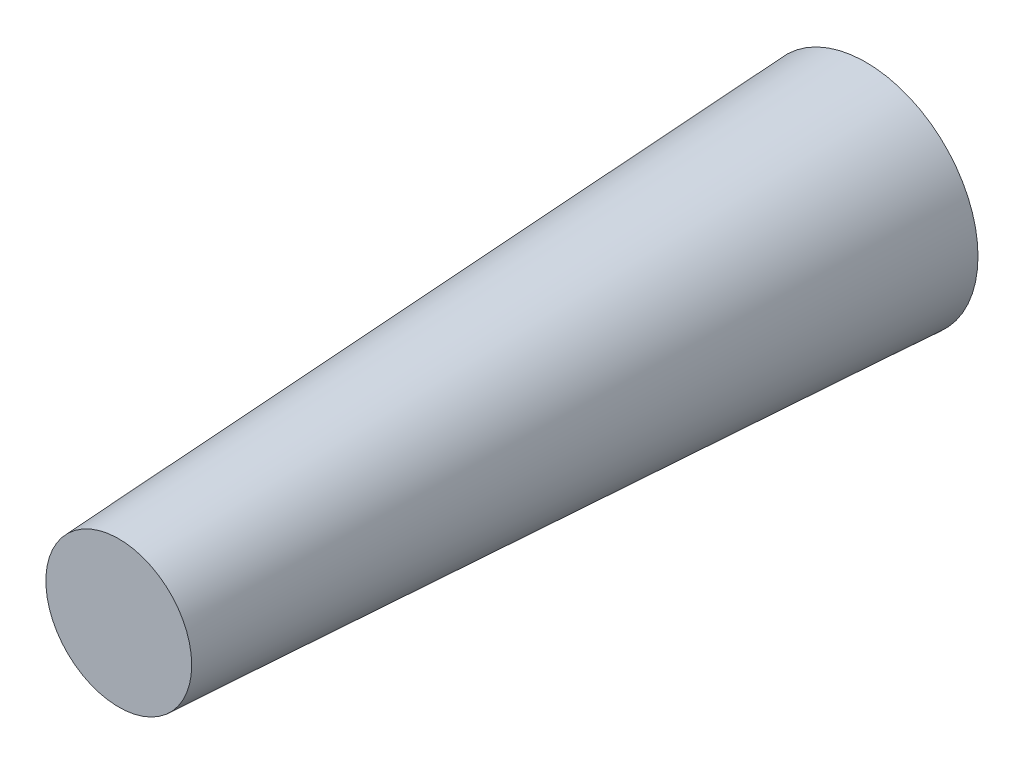
from build123d import *

# Parameters (mm, degrees)
PIN_PROFILE_6_R                   = 3
TAPER_PIN_BODY_20MM_3_DRAFT_DEPTH = 20
TAPER_PIN_BODY_20MM_3_DRAFT_TAPER = 3


with BuildPart() as part:
    # Pin Profile Ø6 → Taper Pin Body 20mm 3° Draft (new body)
    with BuildSketch(Plane.XY):
        Circle(PIN_PROFILE_6_R)
    extrude(amount=TAPER_PIN_BODY_20MM_3_DRAFT_DEPTH, taper=TAPER_PIN_BODY_20MM_3_DRAFT_TAPER)


solid = part.part
